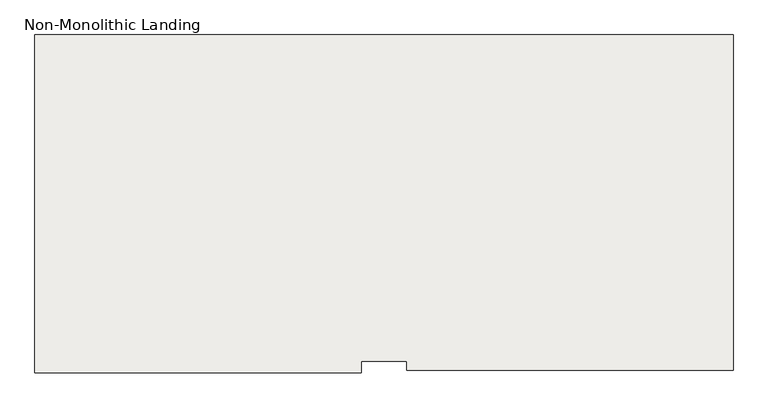
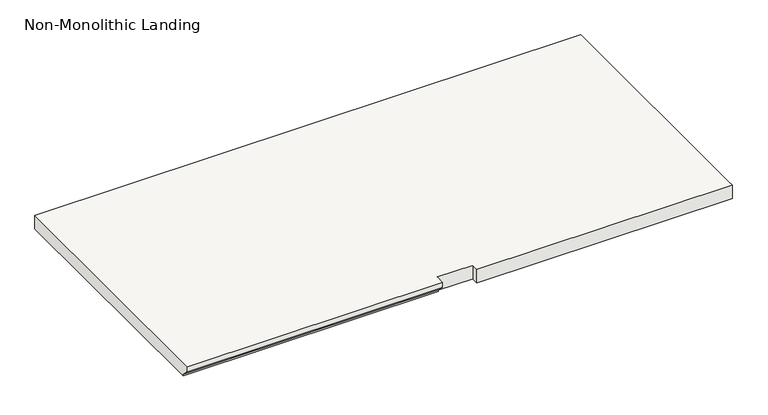
"""IFC4 building model written with IfcOpenShell, lengths in millimetres: slab geometry, Non-Monolithic Landing."""

from ifc_helpers import new_model, si_unit, origin, place, context, project, spatial, faceted_brep, source, transform, mapped, element, save


def non_monolithic_landing_68493687(model_context):
    return source(origin(), model_context, "Body", "Brep", [
        faceted_brep([(-9627.8771954, -2671.4727897, 1504.95), (-9627.8771954, -2671.4727897, 1524.0), (-10542.2771954, -2671.4727897, 1524.0), (-10542.2771954, -2671.4727897, 1504.95), (-9627.8771954, -2646.0727897, 1479.55), (-10542.2771954, -2646.0727897, 1479.55), (-9627.8771954, -2639.7227897, 1524.0), (-9500.8771954, -2639.7227897, 1524.0), (-9500.8771954, -2665.1227897, 1524.0), (-8586.4771954, -2665.1227897, 1524.0), (-8586.4771954, -2639.7227897, 1524.0), (-8586.4771954, -1725.3227897, 1524.0), (-10542.2771954, -1725.3227897, 1524.0), (-9627.8771954, -2646.0727897, 1473.2), (-10542.2771954, -2646.0727897, 1473.2), (-10542.2771954, -1725.3227897, 1473.2), (-8586.4771954, -1725.3227897, 1473.2), (-8586.4771954, -2639.7227897, 1473.2), (-8586.4771954, -2665.1227897, 1473.2), (-9500.8771954, -2665.1227897, 1473.2), (-9500.8771954, -2639.7227897, 1473.2), (-9627.8771954, -2639.7227897, 1473.2)], [[[0, 1, 2, 3]], [[4, 0, 3, 5]], [[6, 7, 8, 9, 10, 11, 12, 2, 1]], [[13, 14, 15, 16, 17, 18, 19, 20, 21]], [[14, 13, 4, 5]], [[6, 1, 0, 4, 13, 21]], [[7, 6, 21, 20]], [[8, 7, 20, 19]], [[9, 8, 19, 18]], [[10, 9, 18, 17]], [[11, 10, 17, 16]], [[12, 11, 16, 15]], [[2, 12, 15, 14, 5, 3]]]),
    ])


if __name__ == "__main__":
    model = new_model("IFC4")
    model_context = context("Model", 3, world=origin())
    ifc_project = project(units=[si_unit("LENGTHUNIT", "METRE", prefix="MILLI")], contexts=[model_context])
    site = spatial("IfcSite", under=ifc_project)
    building = spatial("IfcBuilding", under=site)
    placement = place(None, origin())
    non_monolithic_landing_shape = non_monolithic_landing_68493687(model_context)
    element("IfcSlab", 1, ObjectType="Non-Monolithic Landing", at=placement, inside=building, context=model_context, shape_type="MappedRepresentation", body=[
        mapped(non_monolithic_landing_shape, transform((0.0, 0.0, 0.0), x_axis=(1.0, 0.0, 0.0), y_axis=(0.0, 1.0, 0.0), z_axis=(0.0, 0.0, 1.0))),
    ])
    save(model, "model.ifc")
